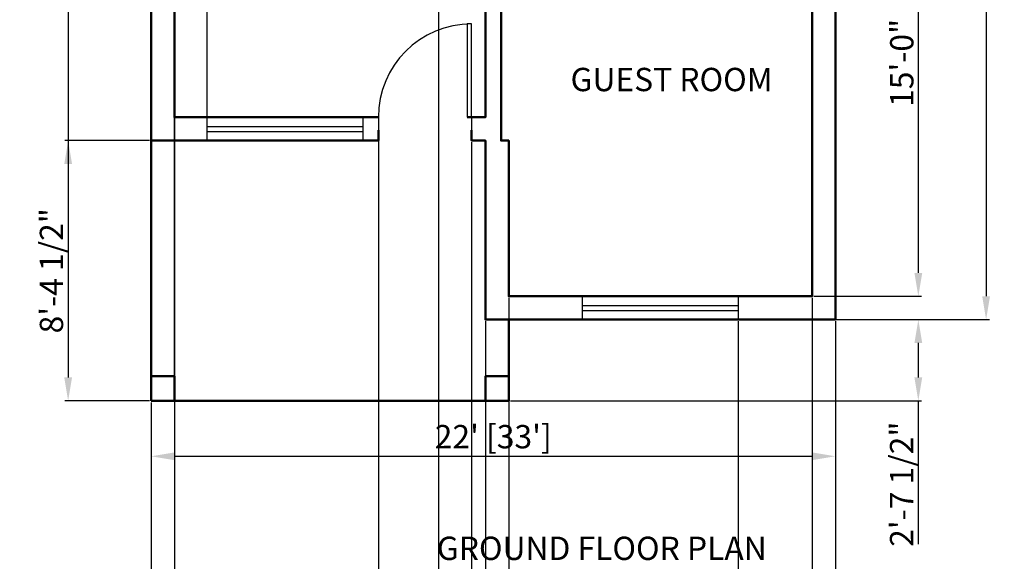
# Model space of a CAD drawing. Units: inches. Extents: x 2429 to 3343, y 1496 to 2530.
# Tile 3 of 7: x 2429 to 2809, y 1910 to 2118. Entities that reach past the tile are written whole.
import ezdxf

# ---------------------------------------------------------------- set-up
doc = ezdxf.new("R2010")
doc.units = ezdxf.units.IN
for name, color, linetype, lineweight in [('A-ANNO-DIMS', 2, 'Continuous', 18), ('A-ANNO-TEXT', 7, 'Continuous', 18), ('A-AREA-IDEN', 3, 'Continuous', 18), ('A-DOOR', 3, 'Continuous', 25), ('A-GLAZ', 4, 'Continuous', 25), ('A-WALL', 7, 'Continuous', 50)]:
    doc.layers.add(name, color=color, linetype=linetype, lineweight=lineweight)
doc.styles.get("Standard").update_dxf_attribs({"font": 'arial.ttf'})
doc.dimstyles.new('ISO-25', dxfattribs={"dimtxt": 9, "dimasz": 9, "dimexe": 1.25, "dimexo": 0.625, "dimtad": 1, "dimdec": 1, "dimlunit": 3, "dimtxsty": 'Standard', "dimcen": 9, "dimadec": 0, "dimazin": 0, "dimtfac": 1, "dimtdec": 1, "dimtmove": 0, "dimatfit": 3, "dimfxl": 1, "dimarcsym": 0})

# ---------------------------------------------------------------- blocks, each defined once
blk = doc.blocks.new('*U2')
for p, q in [((0, 0), (0, -5)), ((-36, 0), (-36, -5))]:
    blk.add_line(p, q)
blk.add_lwpolyline([(0, 0), (0, 36), (-1.75, 36), (-1.75, 0)], close=True)
blk.add_arc((0, 0), 36, 90, 180)
blk = doc.blocks.new('*D5')
at = {"layer": 'A-ANNO-DIMS', "color": 0, "lineweight": -2, "transparency": 16777216}
for p, q in [((2479.77, 1970.81), (2479.77, 1948.8)), ((2743.77, 1970.81), (2743.77, 1948.8)), ((2488.77, 1950.05), (2734.77, 1950.05))]:
    blk.add_line(p, q, dxfattribs=at)
at = {"layer": 'A-ANNO-DIMS', "color": 0, "transparency": 16777216}
for points in [[(2488.77, 1951.55), (2488.77, 1948.55), (2479.77, 1950.05)], [(2734.77, 1951.55), (2734.77, 1948.55), (2743.77, 1950.05)]]:
    blk.add_solid(points, dxfattribs=at)
at = {"layer": 'Defpoints', "color": 0, "transparency": 16777216}
for p in [(2479.77, 1971.44), (2743.77, 1971.44), (2743.77, 1950.05)]:
    blk.add_point(p, dxfattribs=at)
at = {"layer": 'A-ANNO-DIMS', "color": 0, "transparency": 16777216, "insert": (2611.77, 1956.45), "char_height": 9, "attachment_point": 5}
blk.add_mtext("22' [33']", dxfattribs=at)
blk = doc.blocks.new('*D7')
at = {"layer": 'A-ANNO-DIMS', "color": 0, "lineweight": -2, "transparency": 16777216}
for p, q in [((2744.82, 2479.76), (2803.17, 2479.76)), ((2801.92, 2470.76), (2801.92, 2011.75)), ((2744.4, 2002.75), (2803.17, 2002.75))]:
    blk.add_line(p, q, dxfattribs=at)
at = {"layer": 'A-ANNO-DIMS', "color": 0, "transparency": 16777216}
for points in [[(2800.42, 2470.76), (2803.42, 2470.76), (2801.92, 2479.76)], [(2800.42, 2011.75), (2803.42, 2011.75), (2801.92, 2002.75)]]:
    blk.add_solid(points, dxfattribs=at)
at = {"layer": 'Defpoints', "color": 0, "transparency": 16777216}
for p in [(2744.19, 2479.76), (2743.77, 2002.75), (2801.92, 2002.75)]:
    blk.add_point(p, dxfattribs=at)
at = {"layer": 'A-ANNO-DIMS', "color": 0, "transparency": 16777216, "insert": (2795.52, 2241.25), "char_height": 9, "attachment_point": 5, "rotation": 90}
blk.add_mtext('39\'-9" [59\'-7.5"]', dxfattribs=at)
blk = doc.blocks.new('WIN-PLAN-1500')
for p, q in [((3.5, 60), (3.5, 0)), ((5.5, 60), (5.5, 0))]:
    blk.add_line(p, q)
blk.add_lwpolyline([(9, 60), (9, 0), (0, 0), (0, 60)], close=True)
blk = doc.blocks.new('*D29')
at = {"layer": 'A-ANNO-DIMS', "color": 0, "lineweight": -2, "transparency": 16777216}
for p, q in [((2479.15, 2479.76), (2446.52, 2479.76)), ((2447.77, 2470.76), (2447.77, 1980.44)), ((2479.15, 1971.44), (2446.52, 1971.44))]:
    blk.add_line(p, q, dxfattribs=at)
at = {"layer": 'A-ANNO-DIMS', "color": 0, "transparency": 16777216}
for points in [[(2446.27, 2470.76), (2449.27, 2470.76), (2447.77, 2479.76)], [(2446.27, 1980.44), (2449.27, 1980.44), (2447.77, 1971.44)]]:
    blk.add_solid(points, dxfattribs=at)
at = {"layer": 'Defpoints', "color": 0, "transparency": 16777216}
for p in [(2479.77, 2479.76), (2447.77, 1971.44), (2479.77, 1971.44)]:
    blk.add_point(p, dxfattribs=at)
at = {"layer": 'A-ANNO-DIMS', "color": 0, "transparency": 16777216, "insert": (2442.49, 2225.6), "char_height": 9, "attachment_point": 5, "rotation": 90}
blk.add_mtext('42\'-4 1/2"', dxfattribs=at)
blk = doc.blocks.new('*D34')
at = {"layer": 'A-ANNO-DIMS', "color": 0, "lineweight": -2, "transparency": 16777216}
for p, q in [((2590.68, 2320.13), (2590.68, 1870.45)), ((2488.77, 2248.13), (2488.77, 1870.45)), ((2497.77, 1871.7), (2581.68, 1871.7))]:
    blk.add_line(p, q, dxfattribs=at)
at = {"layer": 'A-ANNO-DIMS', "color": 0, "transparency": 16777216}
for points in [[(2497.77, 1873.2), (2497.77, 1870.2), (2488.77, 1871.7)], [(2581.68, 1873.2), (2581.68, 1870.2), (2590.68, 1871.7)]]:
    blk.add_solid(points, dxfattribs=at)
at = {"layer": 'Defpoints', "color": 0, "transparency": 16777216}
for p in [(2590.68, 2320.75), (2488.77, 2248.75), (2590.68, 1871.7)]:
    blk.add_point(p, dxfattribs=at)
at = {"layer": 'A-ANNO-DIMS', "color": 0, "transparency": 16777216, "insert": (2539.73, 1876.92), "char_height": 9, "attachment_point": 5}
blk.add_mtext('8\'-6"', dxfattribs=at)
blk = doc.blocks.new('*D38')
at = {"layer": 'A-ANNO-DIMS', "color": 0, "lineweight": -2, "transparency": 16777216}
for p, q in [((2617.77, 2011.13), (2617.77, 1870.45)), ((2734.77, 2011.13), (2734.77, 1870.45)), ((2626.77, 1871.7), (2725.77, 1871.7))]:
    blk.add_line(p, q, dxfattribs=at)
at = {"layer": 'A-ANNO-DIMS', "color": 0, "transparency": 16777216}
for points in [[(2626.77, 1873.2), (2626.77, 1870.2), (2617.77, 1871.7)], [(2725.77, 1873.2), (2725.77, 1870.2), (2734.77, 1871.7)]]:
    blk.add_solid(points, dxfattribs=at)
at = {"layer": 'Defpoints', "color": 0, "transparency": 16777216}
for p in [(2617.77, 2011.75), (2734.77, 2011.75), (2734.77, 1871.7)]:
    blk.add_point(p, dxfattribs=at)
at = {"layer": 'A-ANNO-DIMS', "color": 0, "transparency": 16777216, "insert": (2676.27, 1876.92), "char_height": 9, "attachment_point": 5}
blk.add_mtext('9\'-9"', dxfattribs=at)
blk = doc.blocks.new('*D39')
at = {"layer": 'A-ANNO-DIMS', "color": 0, "lineweight": -2, "transparency": 16777216}
for p, q in [((2735.4, 2191.75), (2777.02, 2191.75)), ((2775.77, 2182.75), (2775.77, 2020.75)), ((2735.4, 2011.75), (2777.02, 2011.75))]:
    blk.add_line(p, q, dxfattribs=at)
at = {"layer": 'A-ANNO-DIMS', "color": 0, "transparency": 16777216}
for points in [[(2774.27, 2182.75), (2777.27, 2182.75), (2775.77, 2191.75)], [(2774.27, 2020.75), (2777.27, 2020.75), (2775.77, 2011.75)]]:
    blk.add_solid(points, dxfattribs=at)
at = {"layer": 'Defpoints', "color": 0, "transparency": 16777216}
for p in [(2734.77, 2191.75), (2734.77, 2011.75), (2775.77, 2011.75)]:
    blk.add_point(p, dxfattribs=at)
at = {"layer": 'A-ANNO-DIMS', "color": 0, "transparency": 16777216, "insert": (2770.55, 2101.75), "char_height": 9, "attachment_point": 5, "rotation": 90}
blk.add_mtext('15\'-0"', dxfattribs=at)
blk = doc.blocks.new('*D41')
at = {"layer": 'A-ANNO-DIMS', "color": 0, "lineweight": -2, "transparency": 16777216}
for p, q in [((2618.4, 2002.75), (2777.02, 2002.75)), ((2775.77, 1993.75), (2775.77, 1980.44)), ((2618.4, 1971.44), (2777.02, 1971.44)), ((2775.77, 1971.44), (2775.77, 1916.14))]:
    blk.add_line(p, q, dxfattribs=at)
at = {"layer": 'A-ANNO-DIMS', "color": 0, "transparency": 16777216}
for points in [[(2774.27, 1993.75), (2777.27, 1993.75), (2775.77, 2002.75)], [(2774.27, 1980.44), (2777.27, 1980.44), (2775.77, 1971.44)]]:
    blk.add_solid(points, dxfattribs=at)
at = {"layer": 'Defpoints', "color": 0, "transparency": 16777216}
for p in [(2617.77, 2002.75), (2617.77, 1971.44), (2775.77, 1971.44)]:
    blk.add_point(p, dxfattribs=at)
at = {"layer": 'A-ANNO-DIMS', "color": 0, "transparency": 16777216, "insert": (2770.49, 1939.29), "char_height": 9, "attachment_point": 5, "rotation": 90}
blk.add_mtext('2\'-7 1/2"', dxfattribs=at)
blk = doc.blocks.new('*D42')
at = {"layer": 'A-ANNO-DIMS', "color": 0, "lineweight": -2, "transparency": 16777216}
for p, q in [((2479.15, 2071.75), (2446.52, 2071.75)), ((2447.77, 2062.75), (2447.77, 1980.44)), ((2479.15, 1971.44), (2446.52, 1971.44))]:
    blk.add_line(p, q, dxfattribs=at)
at = {"layer": 'A-ANNO-DIMS', "color": 0, "transparency": 16777216}
for points in [[(2446.27, 2062.75), (2449.27, 2062.75), (2447.77, 2071.75)], [(2446.27, 1980.44), (2449.27, 1980.44), (2447.77, 1971.44)]]:
    blk.add_solid(points, dxfattribs=at)
at = {"layer": 'Defpoints', "color": 0, "transparency": 16777216}
for p in [(2479.77, 2071.75), (2447.77, 1971.44), (2479.77, 1971.44)]:
    blk.add_point(p, dxfattribs=at)
at = {"layer": 'A-ANNO-DIMS', "color": 0, "transparency": 16777216, "insert": (2442.49, 2021.59), "char_height": 9, "attachment_point": 5, "rotation": 90}
blk.add_mtext('8\'-4 1/2"', dxfattribs=at)
blk = doc.blocks.new('*D43')
at = {"layer": 'A-ANNO-DIMS', "color": 0, "lineweight": -2, "transparency": 16777216}
for p, q in [((2470.77, 2511.76), (2461.77, 2511.76)), ((2479.77, 1972.06), (2479.77, 2513.01)), ((2479.77, 2511.76), (2488.8, 2511.76)), ((2488.8, 1972.06), (2488.8, 2513.01)), ((2497.8, 2511.76), (2531.97, 2511.76))]:
    blk.add_line(p, q, dxfattribs=at)
at = {"layer": 'A-ANNO-DIMS', "color": 0, "transparency": 16777216}
for points in [[(2470.77, 2513.26), (2470.77, 2510.26), (2479.77, 2511.76)], [(2497.8, 2513.26), (2497.8, 2510.26), (2488.8, 2511.76)]]:
    blk.add_solid(points, dxfattribs=at)
at = {"layer": 'Defpoints', "color": 0, "transparency": 16777216}
for p in [(2488.8, 2511.76), (2479.77, 1971.44), (2488.8, 1971.44)]:
    blk.add_point(p, dxfattribs=at)
at = {"layer": 'A-ANNO-DIMS', "color": 0, "transparency": 16777216, "insert": (2519.38, 2516.98), "char_height": 9, "attachment_point": 5}
blk.add_mtext('0\'-9"', dxfattribs=at)
blk = doc.blocks.new('*D44')
at = {"layer": 'A-ANNO-DIMS', "color": 0, "lineweight": -2, "transparency": 16777216}
for p, q in [((2608.77, 2002.13), (2608.77, 1870.45)), ((2479.77, 1970.81), (2479.77, 1870.45)), ((2488.77, 1871.7), (2599.77, 1871.7))]:
    blk.add_line(p, q, dxfattribs=at)
at = {"layer": 'A-ANNO-DIMS', "color": 0, "transparency": 16777216}
for points in [[(2488.77, 1873.2), (2488.77, 1870.2), (2479.77, 1871.7)], [(2599.77, 1873.2), (2599.77, 1870.2), (2608.77, 1871.7)]]:
    blk.add_solid(points, dxfattribs=at)
at = {"layer": 'Defpoints', "color": 0, "transparency": 16777216}
for p in [(2608.77, 2002.75), (2479.77, 1971.44), (2608.77, 1871.7)]:
    blk.add_point(p, dxfattribs=at)
at = {"layer": 'A-ANNO-DIMS', "color": 0, "transparency": 16777216, "insert": (2544.27, 1876.92), "char_height": 9, "attachment_point": 5}
blk.add_mtext('10\'-9"', dxfattribs=at)
blk = doc.blocks.new('*D45')
at = {"layer": 'A-ANNO-DIMS', "color": 0, "lineweight": -2, "transparency": 16777216}
for p, q in [((2567.44, 2072.42), (2567.44, 1870.45)), ((2603.44, 2071.13), (2603.44, 1870.45)), ((2576.44, 1871.7), (2594.44, 1871.7))]:
    blk.add_line(p, q, dxfattribs=at)
at = {"layer": 'A-ANNO-DIMS', "color": 0, "transparency": 16777216}
for points in [[(2576.44, 1873.2), (2576.44, 1870.2), (2567.44, 1871.7)], [(2594.44, 1873.2), (2594.44, 1870.2), (2603.44, 1871.7)]]:
    blk.add_solid(points, dxfattribs=at)
at = {"layer": 'Defpoints', "color": 0, "transparency": 16777216}
for p in [(2567.44, 2073.04), (2603.44, 2071.75), (2603.44, 1871.7)]:
    blk.add_point(p, dxfattribs=at)
at = {"layer": 'A-ANNO-DIMS', "color": 0, "transparency": 16777216, "insert": (2585.44, 1876.92), "char_height": 9, "attachment_point": 5}
blk.add_mtext('3\'-0"', dxfattribs=at)
blk = doc.blocks.new('*D54')
at = {"layer": 'A-ANNO-DIMS', "color": 0, "lineweight": -2, "transparency": 16777216}
for p, q in [((2479.77, 2072.38), (2479.77, 2513.01)), ((2488.77, 2511.76), (2492.46, 2511.76)), ((2501.46, 2072.38), (2501.46, 2513.01)), ((2501.46, 2511.76), (2555.76, 2511.76))]:
    blk.add_line(p, q, dxfattribs=at)
at = {"layer": 'A-ANNO-DIMS', "color": 0, "transparency": 16777216}
for points in [[(2488.77, 2513.26), (2488.77, 2510.26), (2479.77, 2511.76)], [(2492.46, 2513.26), (2492.46, 2510.26), (2501.46, 2511.76)]]:
    blk.add_solid(points, dxfattribs=at)
at = {"layer": 'Defpoints', "color": 0, "transparency": 16777216}
for p in [(2501.46, 2511.76), (2479.77, 2071.75), (2501.46, 2071.75)]:
    blk.add_point(p, dxfattribs=at)
at = {"layer": 'A-ANNO-DIMS', "color": 0, "transparency": 16777216, "insert": (2533.11, 2517.03), "char_height": 9, "attachment_point": 5}
blk.add_mtext('1\'-9 1/2"', dxfattribs=at)
blk = doc.blocks.new('*D55')
at = {"layer": 'A-ANNO-DIMS', "color": 0, "lineweight": -2, "transparency": 16777216}
for p, q in [((2706.27, 2002.13), (2706.27, 1870.45)), ((2743.77, 2002.13), (2743.77, 1870.45)), ((2715.27, 1871.7), (2734.77, 1871.7)), ((2743.77, 1871.7), (2798.91, 1871.7))]:
    blk.add_line(p, q, dxfattribs=at)
at = {"layer": 'A-ANNO-DIMS', "color": 0, "transparency": 16777216}
for points in [[(2715.27, 1873.2), (2715.27, 1870.2), (2706.27, 1871.7)], [(2734.77, 1873.2), (2734.77, 1870.2), (2743.77, 1871.7)]]:
    blk.add_solid(points, dxfattribs=at)
at = {"layer": 'Defpoints', "color": 0, "transparency": 16777216}
for p in [(2706.27, 2002.75), (2743.77, 2002.75), (2743.77, 1871.7)]:
    blk.add_point(p, dxfattribs=at)
at = {"layer": 'A-ANNO-DIMS', "color": 0, "transparency": 16777216, "insert": (2775.84, 1876.98), "char_height": 9, "attachment_point": 5}
blk.add_mtext('3\'-1 1/2"', dxfattribs=at)

msp = doc.modelspace()

# ---------------------------------------------------------------- linework, layer by layer
at = {"layer": 'A-WALL'}
for p, q in [((2479.77257, 2071.7507), (2479.77257, 1971.43605)), ((2617.77257, 1971.43605), (2617.77257, 2002.7507)), ((2479.77257, 1971.43605), (2617.77257, 1971.43605))]:
    msp.add_line(p, q, dxfattribs=at)
for points in [[(2603.44497, 2075.7507), (2603.44497, 2071.7507), (2608.77257, 2071.7507), (2608.77257, 2002.7507), (2743.77257, 2002.7507), (2743.77257, 2326.7507), (2743.77257, 2479.75602), (2479.77257, 2479.75602), (2479.77257, 2326.7507), (2479.77257, 2320.7507), (2479.77257, 2200.7507), (2479.77257, 2071.7507), (2567.44497, 2071.7507), (2567.44497, 2073.04361), (2567.44497, 2075.7507)], [(2658.07657, 2230.80141), (2656.77257, 2230.80141), (2656.77257, 2256.75602), (2734.77257, 2256.75602), (2734.77257, 2326.7507), (2734.77257, 2368.75602), (2698.77257, 2368.75602), (2698.77257, 2374.75602), (2734.77257, 2374.75602), (2734.77257, 2470.75602), (2488.77257, 2470.75602), (2488.77257, 2326.7507), (2488.77257, 2320.7507), (2488.77257, 2200.7507), (2488.77257, 2080.7507), (2567.44497, 2080.7507)], [(2601.69497, 2080.7507), (2608.77257, 2080.7507), (2608.77257, 2200.7507), (2614.77257, 2200.7507)], [(2614.77257, 2191.7507), (2614.77257, 2071.7507), (2617.77257, 2071.7507), (2617.77257, 2011.7507), (2734.77257, 2011.7507), (2734.77257, 2191.7507), (2650.36679, 2191.7507)]]:
    msp.add_lwpolyline(points, dxfattribs=at)
for points in [[(2479.77257, 1971.43605), (2488.79617, 1971.43605), (2488.79617, 1980.9447), (2479.77257, 1980.9447)], [(2608.74898, 1971.43605), (2617.77257, 1971.43605), (2617.77257, 1980.9447), (2608.74898, 1980.9447)]]:
    msp.add_lwpolyline(points, close=True, dxfattribs=at)

# ---------------------------------------------------------------- block references
at = {"layer": 'A-DOOR'}
msp.add_blockref('*U2', (2603.44497, 2080.7507), dxfattribs=at)
at = {"layer": 'A-GLAZ'}
for p, rotation in [((2561.45789, 2071.75113), 90.00000000000101), ((2706.27293, 2002.75113), 89.99999999999896)]:
    msp.add_blockref('WIN-PLAN-1500', p, dxfattribs=dict(at, rotation=rotation))

# ---------------------------------------------------------------- texts
at = {"layer": 'A-ANNO-TEXT', "insert": (2590, 1919.06231), "char_height": 9, "attachment_point": 1}
msp.add_mtext_dynamic_manual_height_columns('{\\fCalibri|b0|i0|c0|p34;GROUND FLOOR PLAN}', width=142.5053551, gutter_width=12.5, heights=[0], dxfattribs=at)
at = {"layer": 'A-AREA-IDEN', "insert": (2641.59994, 2099.83109), "char_height": 9, "attachment_point": 1}
msp.add_mtext_dynamic_manual_height_columns('{\\fCalibri|b0|i0|c0|p34;GUEST ROOM}', width=82.5181009, gutter_width=12.5, heights=[0], dxfattribs=at)

# ---------------------------------------------------------------- dimensions: what is measured, and where the dimension line sits
at = {"layer": 'A-ANNO-DIMS'}
for base, p1, p2, override, picture, middle in [((2501.45753, 2511.75602), (2479.77257, 2071.7507), (2501.45753, 2071.7507), {"dimdec": 1, "dimlfac": 1, "dimrnd": 0, "dimzin": 1, "dimdsep": 46, "dimlunit": 4, "dimfrac": 2}, '*D54', (2533.10674, 2517.0345)), ((2488.79617, 2511.75602), (2479.77257, 1971.43605), (2488.79617, 1971.43605), {"dimdec": 1, "dimlfac": 1, "dimrnd": 0, "dimzin": 1, "dimdsep": 46, "dimlunit": 4, "dimfrac": 2}, '*D43', (2519.38331, 2516.97617)), ((2590.68041, 1871.69967), (2488.77257, 2248.7507), (2590.68041, 2320.7507), {"dimdec": 1, "dimlfac": 1, "dimrnd": 0, "dimzin": 1, "dimdsep": 46, "dimlunit": 4, "dimfrac": 2}, '*D34', (2539.72649, 1876.91983)), ((2603.44497, 1871.69967), (2567.44497, 2073.04361), (2603.44497, 2071.7507), {"dimdec": 1, "dimlfac": 1, "dimrnd": 0, "dimzin": 1, "dimdsep": 46, "dimlunit": 4, "dimfrac": 2}, '*D45', (2585.44497, 1876.9229)), ((2734.77257, 1871.69967), (2617.77257, 2011.7507), (2734.77257, 2011.7507), {"dimdec": 1, "dimlfac": 1, "dimrnd": 0, "dimzin": 1, "dimdsep": 46, "dimlunit": 4, "dimfrac": 2}, '*D38', (2676.27257, 1876.91983)), ((2608.77257, 1871.69967), (2479.77257, 1971.43605), (2608.77257, 2002.7507), {"dimdec": 1, "dimlfac": 1, "dimrnd": 0, "dimzin": 1, "dimdsep": 46, "dimlunit": 4, "dimfrac": 2}, '*D44', (2544.27257, 1876.91983)), ((2743.77257, 1871.69967), (2706.27257, 2002.7507), (2743.77257, 2002.7507), {"dimdec": 1, "dimlfac": 1, "dimrnd": 0, "dimzin": 1, "dimdsep": 46, "dimlunit": 4, "dimfrac": 2}, '*D55', (2775.84232, 1876.98122)), ((2743.77257, 1950.05317), (2479.77257, 1971.43605), (2743.77257, 1971.43605), {"dimclrd": 0, "dimclre": 0, "dimclrt": 0}, '*D5', (2611.77257, 1956.4459))]:
    dim = msp.add_linear_dim(base=base, p1=p1, p2=p2, dimstyle='ISO-25', override=override, dxfattribs=at)
    dim.commit()
    dim.dimension.update_dxf_attribs({"geometry": picture, "text_midpoint": middle})
for base, p1, p2, override, picture, middle in [((2447.77257, 1971.43605), (2479.77257, 2479.75602), (2479.77257, 1971.43605), {"dimdec": 1, "dimlfac": 1, "dimrnd": 0, "dimzin": 1, "dimdsep": 46, "dimlunit": 4, "dimfrac": 2}, '*D29', (2442.49409, 2225.59604)), ((2801.91709, 2002.7507), (2744.19025, 2479.75602), (2743.77257, 2002.7507), {"dimclrd": 0, "dimclre": 0, "dimclrt": 0}, '*D7', (2795.52436, 2241.25336)), ((2775.77257, 2011.7507), (2734.77257, 2191.7507), (2734.77257, 2011.7507), {"dimdec": 1, "dimlfac": 1, "dimrnd": 0, "dimzin": 1, "dimdsep": 46, "dimlunit": 4, "dimfrac": 2}, '*D39', (2770.55242, 2101.7507)), ((2447.77257, 1971.43605), (2479.77257, 2071.7507), (2479.77257, 1971.43605), {"dimdec": 1, "dimlfac": 1, "dimrnd": 0, "dimzin": 1, "dimdsep": 46, "dimlunit": 4, "dimfrac": 2}, '*D42', (2442.49409, 2021.59338)), ((2775.77257, 1971.43605), (2617.77257, 2002.7507), (2617.77257, 1971.43605), {"dimdec": 1, "dimlfac": 1, "dimrnd": 0, "dimzin": 1, "dimdsep": 46, "dimlunit": 4, "dimfrac": 2}, '*D41', (2770.49409, 1939.2865))]:
    dim = msp.add_linear_dim(base=base, p1=p1, p2=p2, angle=90, dimstyle='ISO-25', override=override, dxfattribs=at)
    dim.commit()
    dim.dimension.update_dxf_attribs({"geometry": picture, "text_midpoint": middle})

doc.saveas('drawing.dxf')
